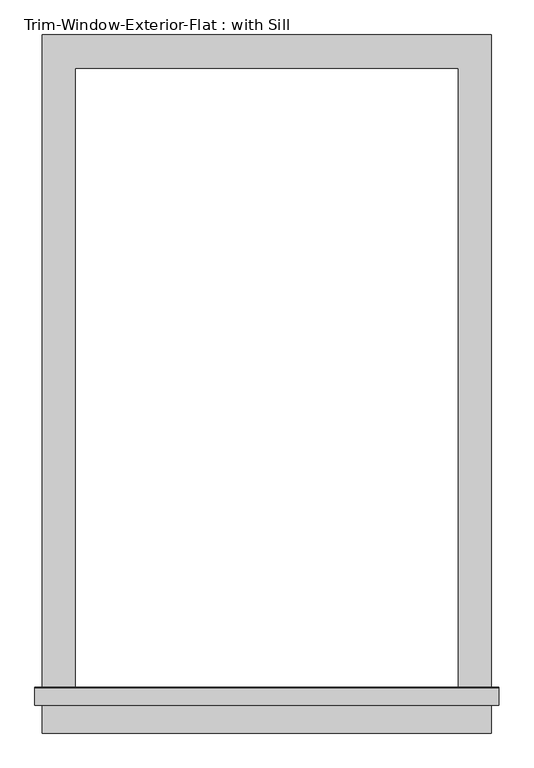
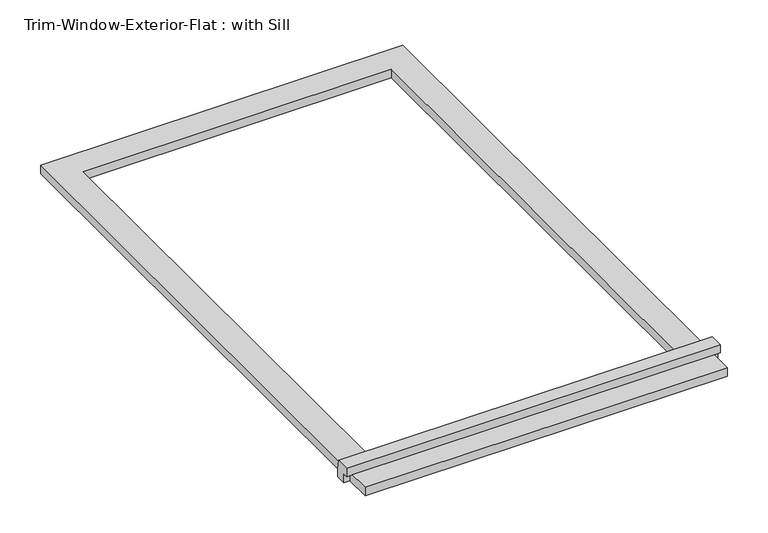
"""IFC4 building model written with IfcOpenShell, lengths in millimetres: proxy geometry, Trim-Window-Exterior-Flat : with Sill."""

from ifc_helpers import new_model, si_unit, frame, origin, origin_with_axes, place, context, project, spatial, polyline, outline, extrude, source, transform, mapped, element, save


def trim_window_exterior_flat_with_sill_e38017c9(model_context):
    return source(origin(), model_context, "Body", "SweptSolid", [
        extrude(outline(polyline([(387.35, -1088.9823709), (387.35, -1146.1323709), (-387.35, -1146.1323709), (-387.35, -1088.9823709), (387.35, -1088.9823709)])), origin_with_axes(), (0.0, 0.0, 1.0), 19.05),
        extrude(outline(polyline([(-1098.55, 38.1), (-1069.2580645, 38.1), (-1066.8, 19.05), (-1066.8, 0.0), (-1088.9823709, 0.0), (-1088.9823709, 19.05), (-1098.55, 19.05), (-1098.55, 38.1)])), frame((-400.05, 0.0, 0.0), z_axis=(1.0, 0.0, 0.0), x_axis=(0.0, 1.0, 0.0)), (0.0, 0.0, 1.0), 800.1),
        extrude(outline(polyline([(-387.35, 57.15), (387.35, 57.15), (387.35, -1066.8), (330.2, -1066.8), (330.2, 0.0), (-330.2, 0.0), (-330.2, -1066.8), (-387.35, -1066.8), (-387.35, 57.15)])), origin_with_axes(), (0.0, 0.0, 1.0), 19.05),
    ])


if __name__ == "__main__":
    model = new_model("IFC4")
    model_context = context("Model", 3, world=origin())
    ifc_project = project(units=[si_unit("LENGTHUNIT", "METRE", prefix="MILLI")], contexts=[model_context])
    site = spatial("IfcSite", under=ifc_project)
    building = spatial("IfcBuilding", under=site)
    placement = place(None, origin())
    trim_window_exterior_flat_with_sill_shape = trim_window_exterior_flat_with_sill_e38017c9(model_context)
    element("IfcBuildingElementProxy", 1, Name="Trim-Window-Exterior-Flat : with Sill", ObjectType="Trim-Window-Exterior-Flat : with Sill", at=placement, inside=building, context=model_context, shape_type="MappedRepresentation", body=[
        mapped(trim_window_exterior_flat_with_sill_shape, transform((0.0, 0.0, 0.0), x_axis=(1.0, 0.0, 0.0), y_axis=(0.0, 1.0, 0.0), z_axis=(0.0, 0.0, 1.0))),
    ])
    save(model, "model.ifc")

# Revit data of these elements
# Type "Trim-Window-Exterior-Flat : with Sill"
#   Trim Width = 0' - 2 1/4"
#   Trim Thickness_Picture Frame = 0' - 1 1/4"
#   Trim Thickness_with Sill = 0' - 0 3/4"
#   Sill Thickness = 0' - 1 1/4"
#   Opening Width [instance default] = 2' - 0"
#   Opening Height [instance default] = 3' - 0"
#   Default Elevation = 4' - 0"
#   Sill = yes
#   Picture Frame = no
#   Trim Material [instance default] = none
# Element 1 (IfcBuildingElementProxy, "Trim-Window-Exterior-Flat : with Sill")
#   Opening Width = 2' - 2"
#   Opening Height = 3' - 6"
#   Trim Material = Clad - White
#   Materials on its faces: "Clad - White"
# Materials
#   "Clad - White": class "Wood", colour RGB 242 242 238, transparency 0, Cost = 0
